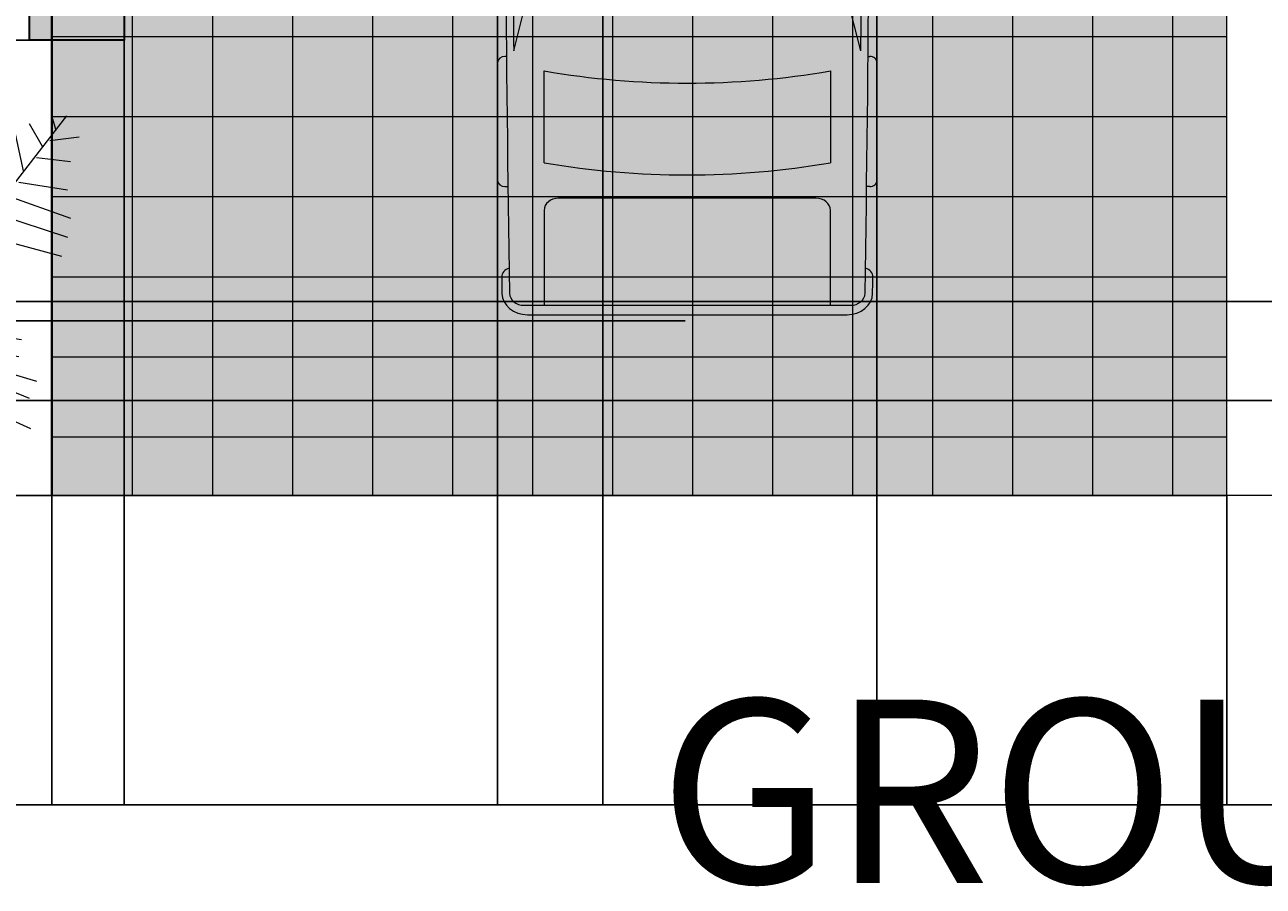
# Model space of a CAD drawing. Units: millimetres. Extents: x -229 to 16545, y -10488 to 4272.
# Tile 1 of 29: x 1930 to 5862, y -10488 to -7754. Entities that reach past the tile are written whole.
import ezdxf

# ---------------------------------------------------------------- set-up
doc = ezdxf.new("R2010")
doc.units = ezdxf.units.MM
for name, color, linetype, lineweight in [('A-ANNO-DIMS', 2, 'Continuous', 18), ('A-ANNO-TEXT', 7, 'Continuous', 25), ('A-COLS', 7, 'Continuous', 35), ('A-WALL', 7, 'Continuous', 35), ('C-PRKG-VEHI', 8, 'Continuous', 18), ('C-PRKG-VEHI-PATT', 252, 'Continuous', 13), ('L-PLNT-TREE', 80, 'Continuous', 18), ('L-PVMT', 7, 'Continuous', 18), ('L-PVMT-JNTS', 8, 'Continuous', 13)]:
    doc.layers.add(name, color=color, linetype=linetype, lineweight=lineweight)
doc.layers.add('L-PVMT-PATT', color=252, linetype='Continuous', lineweight=13, true_color=0x939598)
doc.styles.get("Standard").update_dxf_attribs({"font": 'arial.ttf'})
doc.dimstyles.get("Standard").update_dxf_attribs({"dimtxt": 0.18, "dimasz": 0.18, "dimexe": 0.18, "dimexo": 0.0625, "dimgap": 0.09, "dimtad": 0, "dimtih": 1, "dimtoh": 1, "dimdec": 4, "dimzin": 0, "dimdsep": 46, "dimtxsty": 'Standard', "dimcen": 0.09, "dimadec": 0, "dimazin": 0, "dimtfac": 1, "dimtdec": 4, "dimtofl": 0, "dimtmove": 0, "dimatfit": 3, "dimfxl": 1, "dimtolj": 1, "dimtzin": 0, "dimarcsym": 0})

# ---------------------------------------------------------------- blocks, each defined once
blk = doc.blocks.new('*U18')
for p, q in [((-10.18600000000015, 53.63999999999987), (-13.08399999999983, 55.96199999999976)), ((0, 0), (-10.5, 57)), ((-9.098999999999705, 51.7819999999997), (-6.563000000000101, 55.96199999999976)), ((-8.736999999999625, 47.13799999999969), (-17.06899999999996, 52.71100000000001)), ((-7.65000000000009, 43.42299999999977), (-2.577999999999974, 49.45999999999981)), ((-7.28800000000001, 39.70699999999965), (-21.77800000000025, 46.67299999999977)), ((-5.838999999999941, 35.99199999999973), (4.666999999999916, 48.06699999999977)), ((-5.114000000000032, 27.63199999999983), (10.46300000000019, 46.67299999999977)), ((-5.114000000000032, 28.09699999999975), (-24.67599999999993, 40.63599999999996)), ((-2.940999999999803, 16.48599999999987), (8.652000000000044, 37.84999999999991)), ((-3.665000000000418, 19.27299999999968), (-27.57400000000007, 35.52699999999982)), ((27, 9), (48, 36)), ((27.12699999999995, 9.05600000000004), (31.11200000000008, 35.99199999999973)), ((38.71900000000005, 34.13399999999979), (41.97899999999981, 28.56099999999992)), ((44.15300000000025, 36.45599999999991), (45.23900000000003, 32.74099999999999)), ((16.25900000000001, 5.804999999999836), (23.14199999999983, 31.34799999999973)), ((22.05499999999984, 7.197999999999865), (27.48900000000003, 32.27699999999982)), ((31.83600000000024, 30.88299999999981), (32.56100000000015, 16.48599999999987)), ((35.09600000000001, 32.74099999999999), (37.26999999999998, 22.52399999999989)), ((43.79100000000017, 29.95399999999995), (51.03600000000006, 30.88299999999981)), ((-48.58500000000003, 21.13099999999986), (-49.30899999999974, 29.02600000000007)), ((-43.51299999999992, 28.56099999999992), (-42.42699999999968, 15.55799999999976)), ((-35.54399999999987, 28.09699999999975), (-24.31399999999985, 3.946999999999661)), ((-31.5, 4.5), (-52.5, 25.5)), ((-38.44199999999955, 26.23899999999981), (-34.81899999999996, 7.662999999999783)), ((-14.5329999999999, 2.089999999999918), (-30.83399999999983, 25.30999999999995)), ((-1.128999999999905, 6.733999999999923), (9.014000000000124, 26.70399999999995)), ((3.942000000000007, 1.625), (11.1869999999999, 24.38099999999986)), ((10.10100000000011, 3.482999999999719), (17.70800000000008, 26.23899999999981)), ((40.52999999999975, 25.77499999999986), (48.86200000000008, 24.846)), ((-24.31399999999985, 23.91699999999969), (-2.940999999999803, 13.69999999999982)), ((-47.49800000000004, 19.73699999999962), (-55.83000000000038, 18.34399999999982)), ((36.18300000000045, 19.73699999999962), (48.13699999999972, 17.87999999999988)), ((33.28499999999986, 16.48599999999987), (48.86200000000008, 10.91299999999978)), ((-40.61500000000023, 13.69999999999982), (-55.10500000000002, 10.91299999999978)), ((-20.69099999999981, 13.69999999999982), (-1.128999999999905, 4.875999999999976)), ((29.66199999999981, 12.30699999999979), (48.13699999999972, 6.268999999999778)), ((-33.37000000000035, 6.268999999999778), (-52.20699999999988, 5.339999999999918)), ((0, 0), (27, 9)), ((24.22899999999982, 7.662999999999783), (46.6880000000001, 1.625)), ((-28.29899999999998, 3.482999999999719), (-47.86000000000012, -5.805000000000063)), ((0, 0), (-31.5, 4.5)), ((11.1869999999999, 3.482999999999719), (30.74900000000025, -5.805000000000063)), ((18.06999999999971, 5.804999999999836), (35.09600000000001, -3.483000000000174)), ((-21.41600000000017, 3.017999999999801), (-38.07899999999973, -8.128000000000384)), ((-15.98199999999951, 2.089999999999918), (-30.11000000000013, -9.521000000000186)), ((0, 0), (-22.5, -19.5)), ((-6.563000000000101, 1.161000000000058), (-21.41600000000017, -8.128000000000384)), ((0, 0), (18, -22.5)), ((6.478000000000065, 1.625), (26.03999999999996, -8.592000000000326)), ((2.493000000000392, -3.019000000000005), (-1.490999999999985, -20.20200000000023)), ((1.769000000000232, -2.555000000000063), (24.22899999999982, -9.521000000000186)), ((-6.563000000000101, -5.805000000000063), (-19.96699999999964, -9.985000000000127)), ((-4.751999999999952, -3.483000000000174), (-3.665000000000418, -14.62900000000013)), ((-9.460999999999785, -8.592000000000326), (-6.201000000000021, -23.4530000000002)), ((5.028999999999996, -6.270000000000209), (2.131000000000312, -25.77500000000009)), ((7.564999999999599, -9.056000000000267), (32.19800000000032, -14.62900000000013)), ((-13.44599999999991, -11.37800000000038), (-8.736999999999625, -32.74100000000021)), ((9.014000000000124, -11.37800000000038), (3.579999999999927, -35.99200000000019)), ((-17.43100000000004, -15.09400000000005), (-42.78899999999976, -18.80899999999997)), ((-15.2569999999996, -12.77200000000016), (-30.11000000000013, -12.77200000000016)), ((-17.06899999999996, -15.09400000000005), (-12.721, -40.17200000000025)), ((12.27399999999988, -15.09400000000005), (36.9069999999997, -18.80899999999997)), ((14.08499999999958, -16.95100000000025), (6.478000000000065, -40.17200000000025)), ((-22.5, -19.5), (-37.5, -45)), ((-20.69099999999981, -18.34500000000003), (-17.79300000000012, -44.35200000000032)), ((16.25900000000001, -19.73800000000028), (36.18300000000045, -22.98900000000003)), ((-24.31399999999985, -21.59600000000023), (-42.42699999999968, -22.06000000000017)), ((-25.03800000000001, -23.91800000000035), (-22.86500000000024, -45.28100000000017)), ((18.06999999999971, -22.52400000000012), (8.289000000000215, -45.74500000000012)), ((18, -22.5), (27, -52.5)), ((18.43300000000045, -22.52400000000012), (40.52999999999975, -29.02600000000007)), ((-26.8489999999997, -26.24000000000001), (-40.25300000000015, -25.77500000000009)), ((19.1569999999997, -25.31100000000015), (38.71900000000005, -33.20600000000013)), ((-28.29899999999998, -29.02600000000007), (-42.78899999999976, -31.34800000000018)), ((-29.02300000000014, -30.88400000000002), (-27.93600000000015, -43.88700000000016)), ((20.24400000000014, -30.4190000000001), (15.89699999999993, -44.81600000000026)), ((21.33100000000013, -32.74100000000021), (39.08100000000013, -40.63600000000019)), ((-30.83399999999983, -34.13499999999999), (-42.42699999999968, -35.52800000000025)), ((-32.64600000000019, -36.92100000000005), (-31.92099999999982, -44.35200000000032)), ((22.77999999999975, -37.85000000000014), (19.51900000000023, -48.53200000000015)), ((22.77999999999975, -38.31400000000008), (34.37199999999985, -44.81600000000026)), ((-34.45699999999988, -39.70800000000031), (-40.97800000000006, -42.49400000000014)), ((24.59100000000035, -43.42300000000022), (30.74900000000025, -47.60300000000029)), ((24.59100000000035, -45.74500000000012), (23.14199999999983, -50.85400000000004)), ((26.76400000000012, -49.92500000000018), (28.21300000000019, -50.85400000000004))]:
    blk.add_line(p, q)
blk = doc.blocks.new('*U20')
for p, q in [((46.55368679439944, 38.88847654282876), (22.35054758993934, 38.88847654282876)), ((136.6978032355602, 38.88847654282876), (160.90094244002, 38.88847654282867)), ((21.10406751471477, 37.40863046792069), (21.10406751471477, 36.83230215753705)), ((47.80016686962392, 37.39011648242055), (47.80016686962392, 37.40863046792069)), ((87.98532186932616, 31.87120872459877), (74.75900729854769, 35.92175679182955)), ((134.313356548143, 35.6043097713567), (119.2882629232503, 31.77757799177584)), ((135.4513231603356, 37.07354110333037), (135.4513231603356, 37.40863046792069)), ((162.1474225152445, 37.40863046792049), (162.1474225152445, 36.77402019194128)), ((186.4728846989705, -33.49860931502491), (186.4728846989718, 33.49860931502465)), ((70.0302824853563, 31.53613089391356), (86.40615155322342, 29.35124891408057)), ((188.3990091454065, -32.75868627757393), (188.3990091454077, 32.75868627757058)), ((138.4228833961707, 29.35124891408074), (157.2465674415997, 29.35124891408074)), ((186.4728846989718, 29.35124891408083), (167.0083537481071, 29.35124891408083)), ((164.515393597658, 26.39155676426461), (164.5153935976578, -26.39155676426503)), ((32.26591480791686, 11.62530558863241), (36.12873726252356, 17.16961494239206)), ((36.12873726252356, 17.16961494239206), (50.93891189819171, 17.16961494239206)), ((32.12291633764599, 9.505833383620029), (32.12291633764599, 11.15369945057711)), ((58.9167604809788, -10.77488335095668), (58.9167604809788, 10.77488335095617)), ((66.55009204259746, -10.5288681329018), (66.55009204259746, 10.52886813290129)), ((186.4728846989718, -10.5288681329018), (186.4728846989718, 10.52886813290129)), ((29.77279020470884, 9.505833383620029), (51.68362801571248, 9.505833383620029)), ((82.73706193978568, 8.496039918672748), (82.73706193978568, -8.49603991867258)), ((3.266462181856987, 6.128290093440767), (0.1022408397004821, 0.4060708604429806)), ((-4.43e-14, -2.558e-13), (51.68362801571248, -2.558e-13)), ((0.1022408397004821, -0.4060708604432933), (3.266462181856987, -6.128290093441194)), ((29.77279020470884, -9.50583338362054), (51.68362801571248, -9.50583338362054)), ((32.12291633764599, -9.50583338362054), (32.12291633764599, -11.15369945057762)), ((32.26591480791686, -11.62530558863292), (36.12873726252356, -17.16961494239257)), ((36.12873726252356, -17.16961494239257), (50.93891189819171, -17.16961494239257)), ((86.40615155322318, -29.35124891408145), (70.03028248535594, -31.53613089391442)), ((157.2465674415997, -29.35124891408117), (138.4228833961707, -29.35124891408126)), ((167.008353748107, -29.35124891408126), (186.4728846989707, -29.35124891408108)), ((87.98532186932607, -31.87120872459903), (74.7590072985476, -35.92175679182964)), ((134.3133565481428, -35.60430977135721), (119.2882629232503, -31.77757799177618)), ((21.10406751471477, -37.4086304679212), (21.10406751471477, -36.83230215753756)), ((47.80016686962392, -37.39011648242107), (47.80016686962392, -37.4086304679212)), ((135.4513231603355, -37.07354110333088), (135.4513231603355, -37.4086304679212)), ((162.1474225152445, -37.408630467921), (162.1474225152445, -36.77402019194179)), ((46.55368679439944, -38.88847654282927), (22.35054758993934, -38.88847654282927)), ((136.6978032355602, -38.88847654282927), (160.9009424400199, -38.88847654282918))]:
    blk.add_line(p, q)
for centre, major_axis, ratio, start_param, end_param in [((22.35054758993934, 37.40863046792072), (2.08e-14, -1.479846074908118), 0.842303869543976, 3.141592653589776, 4.712388980384677), ((46.55368679439944, 37.40863046792072), (2.2e-14, 1.479846074908118), 0.8423038695439758, -1.570796326794884, 1.73e-14), ((136.6978032355602, 37.40863046792072), (2.357e-13, -1.479846074908118), 0.842303869543976, 3.141592653589603, 4.712388980384554), ((160.90094244002, 37.40863046792052), (5.59e-14, 1.479846074908118), 0.842303869543976, -1.570796326794865, 4.44e-14), ((266.0300214172791, -27.52442688366631), (1.966072e-10, 313.3077612809058), 0.8423038695435284, 1.367075990158062, 1.391760499156098), ((41.19115208863305, -490.8631038926156), (1.294e-13, 528.2339998381949), 0.8423038695439741, 0.0028100083536837, 0.0755983031096952), ((64.48199294511879, -10555.61767587835), (1.907644e-10, 10593.02630634627), 0.842303869543847, -0.0133969486112073, 0.0027970409639888), ((64.4819929449925, -10555.61767590795), (1.9177683e-09, -10591.54646030096), 0.8423038695482963, 3.133765086725325, 3.140440689641252), ((180.6280394947615, 35.8381667808375), (7.4e-14, 2.219769112362114), 0.8423038695439693, -0.0130174256259048, 1.249894140392862), ((64.48199294754608, -10556.35759891604), (1.349839377e-06, 10595.3130398087), 0.8423038681351469, -0.0133969484821159, -0.0130174254969711), ((183.9799245485226, 33.49860931502124), (3e-16, -2.959692149816168), 0.8423038695439952, 1.570796326796048, 3.128195704978389), ((183.9799245485216, 32.75868627756583), (8.56e-14, -5.246425615115243), 0.8423038695439737, 1.570796326795794, 3.128195704978164), ((135.2911776514449, 5.387441675478555), (2.2715e-12, 81.77258453065997), 0.8423038695439563, 1.245306111696802, 1.507880129813836), ((95.78879860270445, -3666.353346297651), (1.949864e-10, -3698.236159209632), 0.8423038695446962, 3.134048706297306, 3.14409775411291), ((259.1750197310735, -27.52442688366614), (1.506617e-10, -305.3028914627677), 0.8423038695443789, 4.528606069860317, 4.561837674556238), ((37.47375371777758, -593.9621830607928), (6.21e-14, -623.32820996736), 0.8423038695439826, 3.09604606856106, 3.200911180495224), ((134.4003789125686, 5.387441675477674), (4.276e-13, -89.7774543484738), 0.84230386954398, 4.44948196380473, 4.652344057257214), ((149.595361812917, 2.799442537139299), (8.561e-13, -79.57966406425402), 0.842303869543983, 4.372215489277867, 4.640744122441986), ((17.08207736189386, -1.421e-13), (6.87e-14, 147.0179238898305), 0.8423038695439764, 4.511394369635731, 4.913383591133647), ((35.90576140732288, -1.421e-13), (6.87e-14, 147.0179238898305), 0.8423038695439764, 4.511394369635731, 4.913383591133647), ((167.0083537481071, 26.39155676426464), (1.394e-13, 2.959692149816236), 0.842303869543976, 5.55e-14, 1.57079632679492), ((-204.4946649195746, 52.39684969293512), (4.12053e-11, -250.9602162198571), 0.8423038695441164, 1.385369446298923, 1.434372047871027), ((13.03653510440275, 17.00972444508943), (1.2303e-12, 27.41599049210566), 0.8423038695439277, 4.435146050259648, 4.718221029521873), ((14.20086229321332, 17.00972444508943), (1.2303e-12, 27.41599049210566), 0.8423038695439277, 4.435146050259648, 4.718221029521873), ((50.7902773840875, 13.33772416300607), (6.340077547122382, -0.356608581037027), 0.6038335755719145, -1.39555193967809, 1.581314658479915), ((32.74615637525823, 11.15369945057713), (1.313e-13, 0.7399230374541176), 0.8423038695439091, 0.8797135699495516, 1.570796326795045), ((29.77279020470884, -46.66302566589627), (5.12e-14, 56.16885904951626), 0.842303869543976, 7e-16, 0.5903187773915901), ((0.6232400376122422, -1.421e-13), (1e-16, -0.7399230374541245), 0.842303869543842, 4.131459131953847, 5.293318828815531), ((29.77279020470884, 46.66302566589578), (4.004e-13, 56.16885904951626), 0.8423038695439734, 2.55127387619821, 3.141592653589801), ((-204.4946649195746, -52.39684969293552), (4.02945e-11, 250.9602162198562), 0.8423038695441192, -1.43437204787103, -1.385369446298926), ((13.03653510440275, -17.00972444508983), (1.2568e-12, -27.41599049210552), 0.8423038695439318, 1.564964277657711, 1.848039256919935), ((14.20086229321332, -17.00972444508983), (1.2568e-12, -27.41599049210552), 0.8423038695439318, 1.564964277657711, 1.848039256919935), ((149.5953618129329, -2.799442537137565), (4.0897e-12, -79.57966406427697), 0.8423038695439419, -1.499151468852248, -1.230622835688196), ((32.74615637525823, -11.1536994505777), (1.3e-13, -0.7399230374541176), 0.8423038695439093, 4.712388980384541, 5.403471737230034), ((134.4003789125684, -5.387441675478584), (4.2949e-12, -89.77745434847827), 0.8423038695439354, -1.510751403667474, -1.307889310215002), ((135.2911776514465, -5.387441675480715), (3.2038e-12, -81.77258453066244), 0.8423038695439492, -1.50788012981387, -1.245306111696839), ((259.1750197310694, 27.52442688365929), (1.08535e-11, 305.3028914629043), 0.8423038695439974, 1.721347632622872, 1.754579237318777), ((167.008353748107, -26.39155676426503), (1.02e-14, -2.959692149816192), 0.8423038695439885, 4.712388980384686, 6.283185307179581), ((266.0300214172791, 27.52442688366566), (8.75241e-11, 313.3077612806533), 0.8423038695441819, 1.749832154434603, 1.774516663432659), ((37.47375371777847, 593.9621830607904), (1.1693e-12, -623.3282099673584), 0.8423038695439528, -0.0593185269054384, 0.0455465850287298), ((95.78879860271888, 3666.35334629765), (1.637818e-10, -3698.236159209629), 0.8423038695447546, -0.0025051005232382, 0.007543947292366), ((183.9799245485177, -32.7586862775633), (2.428e-13, -5.246425615118353), 0.8423038695439808, 0.0133969486110846, 1.570796326792831), ((183.9799245485216, -33.4986093150211), (9.3e-15, 2.959692149816141), 0.8423038695439732, 3.154989602201626, 4.71238898038339), ((41.19115208863322, 490.8631038926152), (1.37757e-11, -528.2339998381949), 0.8423038695440652, -0.0755983031097181, -0.0028100083537155), ((22.35054758993934, -37.40863046792117), (2.2e-14, 1.479846074908118), 0.8423038695439758, 1.570796326794908, 3.14159265358981), ((64.48199294495228, 10555.61767590795), (6.117947e-10, 10593.02630637587), 0.8423038695458146, 3.138795612625926, 3.154989602201039), ((46.55368679439944, -37.40863046792117), (2.08e-14, -1.479846074908118), 0.842303869543976, -1.69e-14, 1.570796326794884), ((64.48199294503607, 10555.61767590793), (1.6049794e-09, -10591.54646030094), 0.8423038695397146, 0.0011519639481523, 0.0078275668641468), ((136.6978032355602, -37.40863046792109), (1.56e-14, -1.479846074908162), 0.8423038695440105, -1.570796326794875, -1.27e-14), ((160.9009424400199, -37.408630467921), (1.969e-13, 1.479846074908162), 0.8423038695440109, 3.141592653589951, 4.712388980384771), ((180.6280394947581, -35.83816678083949), (2.274e-13, -2.219769112363032), 0.8423038695439803, -1.249894138785958, 0.0130174256254374), ((64.48199294197605, 10556.3575989598), (9.365289701e-07, 10595.31303985772), 0.8423038705260315, 3.154610079306566, 3.154989602290631)]:
    blk.add_ellipse(centre, major_axis=major_axis, ratio=ratio, start_param=start_param, end_param=end_param)
at = {"extrusion": (0, 0, -1)}
blk.add_ellipse((50.7902773840875, -13.33772416300655), major_axis=(6.340077547122382, 0.3566085810370246), ratio=0.6038335755719145, start_param=-1.39555193967809, end_param=1.581314658479915, dxfattribs=at)
blk = doc.blocks.new('COL-300x450')
at = {"transparency": 33554615}
h = blk.add_hatch(color=256, dxfattribs=at)
h.dxf.hatch_style = 1
h.paths.add_polyline_path([(300, 450), (0, 450), (0, 0), (300, 0)])
at = {"transparency": 33554687}
blk.add_lwpolyline([(0, 450), (300, 450), (300, 0), (0, 0)], close=True, dxfattribs=at)
blk = doc.blocks.new('*D47')
at = {"layer": 'A-ANNO-DIMS', "color": 0, "lineweight": -2, "transparency": 16777216}
for p, q in [((912.052246, -9248.334552), (912.0522459999999, -10230.221103)), ((15679.60703, -9248.334552), (15679.60703, -10230.221103)), ((912.2322459999997, -10230.041103), (8295.409228723058, -10230.041103)), ((15679.42703, -10230.041103), (8296.250047276942, -10230.041103))]:
    blk.add_line(p, q, dxfattribs=at)
at = {"layer": 'A-ANNO-DIMS', "color": 0, "transparency": 16777216}
for points in [[(912.2322459999997, -10230.011103), (912.2322459999997, -10230.071103), (912.0522459999999, -10230.041103)], [(15679.42703, -10230.011103), (15679.42703, -10230.071103), (15679.60703, -10230.041103)]]:
    blk.add_solid(points, dxfattribs=at)
at = {"layer": 'Defpoints', "color": 0, "transparency": 16777216}
for p in [(912.052246, -9248.272052), (15679.60703, -9248.272052), (15679.60703, -10230.041103)]:
    blk.add_point(p, dxfattribs=at)
at = {"layer": 'A-ANNO-DIMS', "color": 0, "transparency": 16777216, "insert": (8295.829637999997, -10230.041103), "char_height": 0.18, "attachment_point": 5}
blk.add_mtext('\\A1;14768', dxfattribs=at)
blk = doc.blocks.new('*D58')
at = {"layer": 'A-ANNO-DIMS', "color": 0, "lineweight": -2, "transparency": 16777216}
for p, q in [((2015.933029, -9248.334552), (2015.933029, -10230.221103)), ((5745.933028999999, -9248.334552), (5745.933028999999, -10230.221103)), ((2016.113029, -10230.041103), (3880.574625180082, -10230.041103)), ((5745.753028999999, -10230.041103), (3881.291432819919, -10230.041103))]:
    blk.add_line(p, q, dxfattribs=at)
at = {"layer": 'A-ANNO-DIMS', "color": 0, "transparency": 16777216}
for points in [[(2016.113029, -10230.011103), (2016.113029, -10230.071103), (2015.933029, -10230.041103)], [(5745.753028999999, -10230.011103), (5745.753028999999, -10230.071103), (5745.933028999999, -10230.041103)]]:
    blk.add_solid(points, dxfattribs=at)
at = {"layer": 'Defpoints', "color": 0, "transparency": 16777216}
for p in [(2015.933029, -9248.272052), (5745.933028999999, -9248.272052), (5745.933028999999, -10230.041103)]:
    blk.add_point(p, dxfattribs=at)
at = {"layer": 'A-ANNO-DIMS', "color": 0, "transparency": 16777216, "insert": (3880.933029, -10230.041103), "char_height": 0.18, "attachment_point": 5}
blk.add_mtext('\\A1;3730', dxfattribs=at)
blk = doc.blocks.new('*D62')
at = {"layer": 'A-ANNO-DIMS', "color": 0, "lineweight": -2, "transparency": 16777216}
for p, q in [((5745.870529000002, -4748.272052000002), (-228.8374730000013, -4748.272052000003)), ((-228.6574730000007, -4748.452052000003), (-228.6574730000002, -6998.090148862215)), ((-228.6574729999998, -9248.092052000005), (-228.6574730000002, -6998.453955137795)), ((5745.870529000002, -9248.272052000004), (-228.8374730000003, -9248.272052000006))]:
    blk.add_line(p, q, dxfattribs=at)
at = {"layer": 'A-ANNO-DIMS', "color": 0, "transparency": 16777216}
for points in [[(-228.6874730000008, -4748.452052000003), (-228.6274730000008, -4748.452052000003), (-228.6574730000007, -4748.272052000003)], [(-228.6874729999997, -9248.092052000005), (-228.6274729999997, -9248.092052000005), (-228.6574729999998, -9248.272052000006)]]:
    blk.add_solid(points, dxfattribs=at)
at = {"layer": 'Defpoints', "color": 0, "transparency": 16777216}
for p in [(5745.933029000002, -4748.272052000002), (-228.6574729999998, -9248.272052000006), (5745.933029000002, -9248.272052000004)]:
    blk.add_point(p, dxfattribs=at)
at = {"layer": 'A-ANNO-DIMS', "color": 0, "transparency": 16777216, "insert": (-228.6574730000022, -6998.272052000003), "char_height": 0.18, "attachment_point": 5}
blk.add_mtext('\\A1;4500', dxfattribs=at)
blk = doc.blocks.new('*D91')
at = {"layer": 'A-ANNO-DIMS', "color": 0, "lineweight": -2, "transparency": 16777216}
for p, q in [((2245.933029, -4748.334552), (2245.933028999999, -10230.221103)), ((3765.491243, -4748.334552), (3765.491243, -10230.221103)), ((2246.113028999999, -10230.041103), (3005.257040502046, -10230.041103)), ((3765.311243, -10230.041103), (3006.167231497953, -10230.041103))]:
    blk.add_line(p, q, dxfattribs=at)
at = {"layer": 'A-ANNO-DIMS', "color": 0, "transparency": 16777216}
for points in [[(2246.113028999999, -10230.011103), (2246.113028999999, -10230.071103), (2245.933028999999, -10230.041103)], [(3765.311243, -10230.011103), (3765.311243, -10230.071103), (3765.491243, -10230.041103)]]:
    blk.add_solid(points, dxfattribs=at)
at = {"layer": 'Defpoints', "color": 0, "transparency": 16777216}
for p in [(2245.933029, -4748.272051999999), (3765.491243, -4748.272051999999), (3765.491243, -10230.041103)]:
    blk.add_point(p, dxfattribs=at)
at = {"layer": 'A-ANNO-DIMS', "color": 0, "transparency": 16777216, "insert": (3005.712136, -10230.041103), "char_height": 0.18, "attachment_point": 5}
blk.add_mtext('\\A1;1519.6', dxfattribs=at)
blk = doc.blocks.new('*D92')
at = {"layer": 'A-ANNO-DIMS', "color": 0, "lineweight": -2, "transparency": 16777216}
for p, q in [((1945.870529000001, -7803.015189000004), (-228.8374730000004, -7803.015189000004)), ((-228.6574730000004, -7803.195189000004), (-228.6574730000002, -8525.461655970674)), ((-228.6574730000001, -9248.092052000004), (-228.6574730000002, -8525.825585029335)), ((2015.870529000001, -9248.272052000004), (-228.8374729999999, -9248.272052000004))]:
    blk.add_line(p, q, dxfattribs=at)
at = {"layer": 'A-ANNO-DIMS', "color": 0, "transparency": 16777216}
for points in [[(-228.6874730000004, -7803.195189000004), (-228.6274730000004, -7803.195189000004), (-228.6574730000004, -7803.015189000004)], [(-228.6874730000001, -9248.092052000004), (-228.6274730000001, -9248.092052000004), (-228.6574730000001, -9248.272052000004)]]:
    blk.add_solid(points, dxfattribs=at)
at = {"layer": 'Defpoints', "color": 0, "transparency": 16777216}
for p in [(1945.933029000001, -7803.015189000004), (-228.6574730000001, -9248.272052000004), (2015.933029000001, -9248.272052000004)]:
    blk.add_point(p, dxfattribs=at)
at = {"layer": 'A-ANNO-DIMS', "color": 0, "transparency": 16777216, "insert": (-228.6574730000026, -8525.643620500003), "char_height": 0.18, "attachment_point": 5}
blk.add_mtext('\\A1;1445.3', dxfattribs=at)
blk = doc.blocks.new('*D95')
at = {"layer": 'A-ANNO-DIMS', "color": 0, "lineweight": -2, "transparency": 16777216}
for p, q in [((3431.620292, -6103.680351), (3431.620292, -10230.221103)), ((4635.562560999999, -6103.680351), (4635.562560999999, -10230.221103)), ((3431.800292, -10230.041103), (4033.241494712823, -10230.041103)), ((4635.382560999999, -10230.041103), (4033.941358287175, -10230.041103))]:
    blk.add_line(p, q, dxfattribs=at)
at = {"layer": 'A-ANNO-DIMS', "color": 0, "transparency": 16777216}
for points in [[(3431.800292, -10230.011103), (3431.800292, -10230.071103), (3431.620292, -10230.041103)], [(4635.382560999999, -10230.011103), (4635.382560999999, -10230.071103), (4635.562560999999, -10230.041103)]]:
    blk.add_solid(points, dxfattribs=at)
at = {"layer": 'Defpoints', "color": 0, "transparency": 16777216}
for p in [(3431.620292, -6103.617851), (4635.562560999999, -6103.617851), (4635.562560999999, -10230.041103)]:
    blk.add_point(p, dxfattribs=at)
at = {"layer": 'A-ANNO-DIMS', "color": 0, "transparency": 16777216, "insert": (4033.591426499999, -10230.041103), "char_height": 0.18, "attachment_point": 5}
blk.add_mtext('\\A1;1204', dxfattribs=at)
blk = doc.blocks.new('*D96')
at = {"layer": 'A-ANNO-DIMS', "color": 0, "lineweight": -2, "transparency": 16777216}
for p, q in [((4033.528927000001, -5757.644295000002), (-228.8374730000011, -5757.644295000003)), ((-228.6574730000006, -5757.824295000003), (-228.6574730000002, -7225.597539470673)), ((-228.6574729999999, -8693.734713000003), (-228.6574730000002, -7225.961468529336)), ((4027.243185000002, -8693.914713000004), (-228.837473, -8693.914713000004))]:
    blk.add_line(p, q, dxfattribs=at)
at = {"layer": 'A-ANNO-DIMS', "color": 0, "transparency": 16777216}
for points in [[(-228.6874730000005, -5757.824295000003), (-228.6274730000005, -5757.824295000003), (-228.6574730000006, -5757.644295000003)], [(-228.6874729999999, -8693.734713000003), (-228.6274729999999, -8693.734713000003), (-228.6574729999999, -8693.914713000004)]]:
    blk.add_solid(points, dxfattribs=at)
at = {"layer": 'Defpoints', "color": 0, "transparency": 16777216}
for p in [(4033.591427000001, -5757.644295000002), (-228.6574729999999, -8693.914713000004), (4027.305685000001, -8693.914713000004)]:
    blk.add_point(p, dxfattribs=at)
at = {"layer": 'A-ANNO-DIMS', "color": 0, "transparency": 16777216, "insert": (-228.6574730000022, -7225.779504000001), "char_height": 0.18, "attachment_point": 5}
blk.add_mtext('\\A1;2936', dxfattribs=at)
blk = doc.blocks.new('*D98')
at = {"layer": 'A-ANNO-DIMS', "color": 0, "lineweight": -2, "transparency": 16777216}
for p, q in [((5975.870529000001, -8632.301380000004), (-228.8374730000005, -8632.301380000006)), ((-228.6574730000003, -8632.481380000007), (-228.6574730000002, -8789.345922470675)), ((-228.6574730000002, -8946.574394000005), (-228.6574730000002, -8789.709851529336)), ((5975.870529000001, -8946.754394000001), (-228.8374730000004, -8946.754394000007))]:
    blk.add_line(p, q, dxfattribs=at)
at = {"layer": 'A-ANNO-DIMS', "color": 0, "transparency": 16777216}
for points in [[(-228.6874730000003, -8632.481380000007), (-228.6274730000003, -8632.481380000007), (-228.6574730000003, -8632.301380000006)], [(-228.6874730000002, -8946.574394000005), (-228.6274730000002, -8946.574394000005), (-228.6574730000002, -8946.754394000007)]]:
    blk.add_solid(points, dxfattribs=at)
at = {"layer": 'Defpoints', "color": 0, "transparency": 16777216}
for p in [(-228.6574730000003, -8632.301380000006), (5975.933029000001, -8632.301380000004), (5975.933029000001, -8946.754394000001)]:
    blk.add_point(p, dxfattribs=at)
at = {"layer": 'A-ANNO-DIMS', "color": 0, "transparency": 16777216, "insert": (-228.6574730000027, -8789.527887000004), "char_height": 0.18, "attachment_point": 5}
blk.add_mtext('\\A1;314.45', dxfattribs=at)

msp = doc.modelspace()

# ---------------------------------------------------------------- hatches: boundary and pattern name
at = {"layer": 'C-PRKG-VEHI-PATT'}
h = msp.add_hatch(color=256, dxfattribs=at)
h.dxf.hatch_style = 1
edge = h.paths.add_edge_path()
edge.add_ellipse((3607.529211185457, -9769.523765348671), major_axis=(4725.912256580008, 3.0749239e-09), ratio=0.8423038695445281, start_angle=77.5553727065174, end_angle=79.7904610028182)
edge.add_ellipse((4844.664368095724, -2592.185106036592), major_axis=(3884.719060684347, 1.125906e-09), ratio=0.8423038695442183, start_angle=257.4450673558462, end_angle=260.74343399278183, ccw=False)
edge.add_line((4128.453814510914, -5808.20724164565), (4039.87716894264, -5759.226924584826))
edge.add_ellipse((4033.591426782733, -5767.29169096579), major_axis=(11.45358085171419, 4.4945e-12), ratio=0.8423038695438549, start_angle=52.06686954012766, end_angle=89.99999999999291)
edge.add_line((4033.59142678273, -5757.644295494259), (4033.59142678273, -5810.864491195777))
edge.add_ellipse((3311.274766540754, -6218.509875466019), major_axis=(-869.4614654596021, 1.80077e-11), ratio=0.8423038695439853, start_angle=180.0000000000011, end_angle=209.4385695979805, ccw=False)
edge.add_line((4180.736232000355, -6218.50987546602), (4180.736232000355, -6254.888469336996))
edge.add_line((4180.736232000355, -6254.888469336996), (4208.936604088284, -6254.888469336996))
edge.add_ellipse((4206.244246044127, -6264.535864808529), major_axis=(-11.45358085171833, 5.0922e-12), ratio=0.8423038695436069, start_angle=225.5197891174528, end_angle=270.00000000002547, ccw=False)
edge.add_line((4213.544436413884, -6257.102002985786), (4299.367139905714, -6316.896261388502))
edge.add_line((4299.367139905714, -6316.896261388502), (4299.367139905714, -6546.149202615045))
edge.add_ellipse((4240.051685953036, -6543.848426266054), major_axis=(5.520094670108304, 98.1407350715287), ratio=0.6038335755718915, start_angle=106.3425919543132, end_angle=270.99798572498946, ccw=False)
edge.add_line((4180.736232000355, -6557.67697757519), (4180.736232000355, -6218.50987546602))
edge.add_ellipse((3311.274766540754, -6218.509875466019), major_axis=(-869.4614654596021, 1.80077e-11), ratio=0.8423038695439853, start_angle=180.0000000000011, end_angle=209.4385695979805)
edge.add_ellipse((4755.908087024709, -6218.50987546602), major_axis=(869.4614654596019, 1.2409e-11), ratio=0.842303869543984, start_angle=150.5614304020198, end_angle=179.9999999999992)
edge.add_line((3886.446621565107, -6218.509875466021), (3886.446621565105, -6557.676977575214))
edge.add_ellipse((3827.131167612427, -6543.848426266054), major_axis=(-5.520094670108304, 98.1407350715287), ratio=0.6038335755718915, start_angle=89.0020142750106, end_angle=253.6574080456868, ccw=False)
edge.add_line((3767.815713659748, -6546.149202615045), (3767.815713659748, -6316.896261388502))
edge.add_line((3767.815713659748, -6316.896261388502), (3855.713030733728, -6255.656581488097))
edge.add_ellipse((3860.938607521334, -6264.535864808529), major_axis=(-11.45358085171114, 2.4167e-12), ratio=0.842303869544136, start_angle=-89.99999999998789, end_angle=-45.51978911742532, ccw=False)
edge.add_line((3860.938607521328, -6254.888469336996), (3886.446621565107, -6254.888469336996))
edge.add_line((3886.446621565107, -6254.888469336996), (3886.446621565107, -6218.509875466018))
edge.add_ellipse((4755.908087024709, -6218.50987546602), major_axis=(869.4614654596019, 1.2409e-11), ratio=0.842303869543984, start_angle=150.5614304020199, end_angle=179.9999999999992, ccw=False)
edge.add_line((4033.59142678273, -5810.86449119578), (4033.59142678273, -5757.644295494258))
edge.add_ellipse((4033.591426782733, -5767.29169096579), major_axis=(11.45358085171419, 4.4945e-12), ratio=0.8423038695438549, start_angle=89.99999999999291, end_angle=127.9331304598159)
edge.add_line((4027.305684622828, -5759.226924584826), (3938.729039054555, -5808.207241645646))
edge.add_ellipse((3222.518485469741, -2592.185106036592), major_axis=(3884.719060685492, 7.18321e-11), ratio=0.8423038695439776, start_angle=-80.74343399279951, end_angle=-77.44506735586378, ccw=False)
edge.add_ellipse((4459.653642379904, -9769.523765348607), major_axis=(4725.912256583255, 9.99789e-11), ratio=0.8423038695439494, start_angle=100.2095389971419, end_angle=102.4446272934428)
edge.add_ellipse((13227.78263612094, -6337.716338528086), major_axis=(9648.760328614822, 3.05852e-11), ratio=0.8423038695439373, start_angle=177.1362853921621, end_angle=182.1985405659548)
edge.add_ellipse((3950.196944261551, -7838.084460829144), major_axis=(1389.703090715241, 7.69205e-11), ratio=0.842303869543924, start_angle=94.082410691147, end_angle=107.71995322274691, ccw=False)
edge.add_line((3866.802461740376, -6669.641686482127), (4200.380391825095, -6669.641686482127))
edge.add_ellipse((4116.985909303905, -7838.084460829148), major_axis=(1389.703090715146, 5.3309e-12), ratio=0.8423038695439844, start_angle=72.28004677724942, end_angle=85.91758930884919, ccw=False)
edge.add_ellipse((-5160.599782555511, -6337.716338528068), major_axis=(9648.76032861485, 3.05852e-11), ratio=0.8423038695439409, start_angle=-2.198540565955437, end_angle=2.863714607837381)
edge = h.paths.add_edge_path()
edge.add_ellipse((-159361.2677283546, -6755.788267626439), major_axis=(-163973.9231279127, 1.03867551e-08), ratio=0.8423038695433289, start_angle=179.6161332212111, end_angle=180.0902290885979)
edge.add_ellipse((-159361.2677283546, -6755.788267626439), major_axis=(-163973.9231279127, 1.03867551e-08), ratio=0.8423038695433289, start_angle=180.0902290885979, end_angle=180.1349865768619)
edge.add_ellipse((-3564.68564119695, -6395.259516187628), major_axis=(-8176.756932164527, 2.256357e-10), ratio=0.8423038695440322, start_angle=180.1356123904399, end_angle=182.1799503136467)
edge.add_ellipse((-3564.68564119695, -6395.259516187628), major_axis=(-8176.756932164527, 2.256357e-10), ratio=0.8423038695440322, start_angle=182.1799503136467, end_angle=183.6504275857005)
edge.add_ellipse((3607.529211185454, -9875.635228402642), major_axis=(4849.823013544719, 2.3877334e-09), ratio=0.8423038695443318, start_angle=76.21947101047385, end_angle=77.87403444768762)
edge.add_ellipse((-5160.599782555511, -6337.716338528068), major_axis=(9648.76032861485, 3.05852e-11), ratio=0.8423038695439409, start_angle=-2.1985405659553976, end_angle=2.8637146078373803, ccw=False)
edge.add_ellipse((4116.985909303905, -7838.084460829148), major_axis=(1389.703090715146, 5.3309e-12), ratio=0.8423038695439844, start_angle=72.28004677724944, end_angle=85.91758930884916)
edge.add_line((4200.380391825095, -6669.641686482127), (3866.802461740375, -6669.641686482127))
edge.add_ellipse((3950.196944261551, -7838.084460829144), major_axis=(1389.703090715241, 7.69205e-11), ratio=0.842303869543924, start_angle=94.08241069114707, end_angle=107.7199532227469)
edge.add_ellipse((13227.78263612094, -6337.716338528086), major_axis=(9648.760328614822, 3.05852e-11), ratio=0.8423038695439373, start_angle=177.1362853921622, end_angle=182.1985405659549, ccw=False)
edge.add_ellipse((4459.653642380003, -9875.635228402642), major_axis=(4849.823013547592, 8.133391e-10), ratio=0.8423038695438513, start_angle=102.1259655522744, end_angle=103.7805289894881)
edge.add_ellipse((11631.86849476242, -6395.259516187635), major_axis=(8176.756932164531, 1.784299e-10), ratio=0.8423038695440094, start_angle=176.3495724142996, end_angle=177.8200496863535)
edge.add_ellipse((11631.86849476242, -6395.259516187635), major_axis=(8176.756932164531, 1.784299e-10), ratio=0.8423038695440094, start_angle=177.8200496863535, end_angle=179.8643876095602)
edge.add_ellipse((167428.4505823782, -6755.788267623933), major_axis=(-163973.9231283709, 3.9422692e-09), ratio=0.8423038695444919, start_angle=-0.1349865768556417, end_angle=-0.0902290885918171)
edge.add_ellipse((167428.4505823782, -6755.788267623933), major_axis=(-163973.9231283709, 3.9422692e-09), ratio=0.8423038695444919, start_angle=-0.0902290885918171, end_angle=0.3838667787936917)
edge.add_ellipse((167428.4505823782, -6755.788267623933), major_axis=(-163973.9231283709, 3.9422692e-09), ratio=0.8423038695444919, start_angle=0.3838667787936917, end_angle=0.5282714718187317)
edge.add_ellipse((167428.4505823782, -6755.788267623933), major_axis=(-163973.9231283709, 3.9422692e-09), ratio=0.8423038695444919, start_angle=0.5282714718187317, end_angle=0.6465540970623085)
edge.add_ellipse((3515.052320972862, -8605.547164094223), major_axis=(45.81432340685111, 4.6009e-12), ratio=0.8423038695439874, start_angle=180.6465540970845, end_angle=269.9999999999056)
edge.add_line((3515.052320972781, -8644.136745980357), (3579.251062286293, -8644.136745980357))
edge.add_line((3579.251062286293, -8644.136745980357), (3579.25106228629, -8338.779260567762))
edge.add_ellipse((3625.065385693143, -8342.837059794769), major_axis=(-45.81432340685263, 1.5796e-12), ratio=0.8423038695439878, start_angle=-89.9999999999979, end_angle=1.9895196601282805e-12, ccw=False)
edge.add_line((3625.065385693143, -8304.247477908637), (4446.934968270596, -8304.247477908639))
edge.add_ellipse((4442.11746787232, -8342.837059794772), major_axis=(-45.81432340685263, 2.8e-15), ratio=0.842303869543988, start_angle=180, end_angle=270, ccw=False)
edge.add_line((4487.931791279172, -8342.837059794772), (4487.931791279172, -8644.136745980375))
edge.add_line((4487.931791279172, -8644.136745980373), (4552.130532592662, -8644.136745980375))
edge.add_ellipse((4552.130532592609, -8605.547164094241), major_axis=(-45.81432340685346, 1.7729e-12), ratio=0.8423038695439725, start_angle=90.000000000083, end_angle=179.3534459029321)
edge.add_ellipse((-159361.2677283546, -6755.788267626439), major_axis=(-163973.9231279127, 1.03867551e-08), ratio=0.8423038695433289, start_angle=179.3534459029417, end_angle=179.3813568036844)
edge.add_ellipse((-159361.2677283546, -6755.788267626439), major_axis=(-163973.9231279127, 1.03867551e-08), ratio=0.8423038695433289, start_angle=179.3813568036844, end_angle=179.4717285281857)
edge.add_ellipse((-159361.2677283546, -6755.788267626439), major_axis=(-163973.9231279127, 1.03867551e-08), ratio=0.8423038695433289, start_angle=179.4717285281857, end_angle=179.6161332212111)
edge = h.paths.add_edge_path(flags=16)
edge.add_ellipse((-52719.43876303247, -7240.399519955929), major_axis=(57246.55770143846, 8.170279e-10), ratio=0.842303869544162, start_angle=-0.3640763488911554, end_angle=0.1208973690318383)
edge.add_line((4526.939312293975, -7119.606211509014), (4589.639454651214, -6914.870508417749))
edge.add_ellipse((-159361.2677288128, -6755.788267624483), major_axis=(163951.0159666675, 3.23007761e-08), ratio=0.842303869549042, start_angle=-0.37776419392122307, end_angle=-0.055594313510596294, ccw=False)
edge.add_line((4584.725558298378, -7836.737404937529), (4525.48996268015, -7604.157642007916))
edge = h.paths.add_edge_path(flags=16)
edge.add_line((4165.105212949923, -7038.366181950441), (3902.077640615548, -7038.366181950441))
edge.add_ellipse((3990.257674735825, -8073.294011525872), major_axis=(1231.84719271423, 3.9463e-11), ratio=0.8423038695439561, start_angle=94.87006959713399, end_angle=112.7919148775847)
edge.add_line((3579.251062286288, -7095.161567973676), (3545.430352373573, -6841.672582103935))
edge.add_ellipse((3950.196944261518, -7851.873510313874), major_axis=(1265.792333751566, 7.14673e-11), ratio=0.8423038695439378, start_angle=94.2774209630507, end_angle=111.8349537967049, ccw=False)
edge.add_line((3870.610635088292, -6787.801246035458), (4196.572218477172, -6787.801246035458))
edge.add_ellipse((4116.985909303919, -7851.87351031385), major_axis=(1265.792333751468, 7.9473e-12), ratio=0.8423038695439835, start_angle=68.16504620328988, end_angle=85.72257903694413, ccw=False)
edge.add_line((4521.752501191884, -6841.672582103939), (4487.931791279168, -7095.16156797368))
edge.add_ellipse((4076.925178829671, -8073.294011525625), major_axis=(1231.847192713881, 3.61807e-11), ratio=0.8423038695439931, start_angle=67.20808512240832, end_angle=85.12993040286263)
edge = h.paths.add_edge_path(flags=16)
edge.add_ellipse((4033.591426782733, -6022.064977478797), major_axis=(-2275.752467063544, 5.6979e-12), ratio=0.8423038695439709, start_angle=76.4018653097695, end_angle=103.5981346902307)
edge.add_line((4487.931791279172, -7900.350504724528), (4487.931791279172, -8191.730251303665))
edge.add_ellipse((4033.591426782733, -6313.444724057934), major_axis=(2275.752467063524, 1.15e-12), ratio=0.8423038695439785, start_angle=256.4018653097693, end_angle=283.5981346902305, ccw=False)
edge.add_line((3579.25106228629, -8191.730251303662), (3579.25106228629, -7900.350504724527))
edge = h.paths.add_edge_path(flags=16)
edge.add_line((3541.69289088531, -7604.157642007925), (3482.457295267053, -7836.737404937647))
edge.add_ellipse((167428.450582378, -6755.788267625229), major_axis=(163951.0159666672, 1.7265743e-08), ratio=0.842303869542198, start_angle=180.055594313493, end_angle=180.3777641939035, ccw=False)
edge.add_line((3477.543398914246, -6914.870508417725), (3540.243541271509, -7119.606211509064))
edge.add_ellipse((60786.62161659793, -7240.399519956177), major_axis=(-57246.55770143843, 1.560408e-10), ratio=0.8423038695499789, start_angle=-0.1208973690328125, end_angle=0.364076348890219)
h = msp.add_hatch(color=256, dxfattribs=at)
h.dxf.hatch_style = 1
edge = h.paths.add_edge_path()
edge.add_ellipse((4116.985909303919, -7851.87351031385), major_axis=(1265.792333751468, 7.9473e-12), ratio=0.8423038695439835, start_angle=68.1650462032899, end_angle=85.72257903694413)
edge.add_line((4196.572218477172, -6787.801246035458), (3870.610635088292, -6787.801246035458))
edge.add_ellipse((3950.196944261518, -7851.873510313874), major_axis=(1265.792333751566, 7.14673e-11), ratio=0.8423038695439378, start_angle=94.27742096305064, end_angle=111.8349537967049)
edge.add_line((3545.430352373573, -6841.672582103933), (3579.251062286288, -7095.161567973675))
edge.add_ellipse((3990.257674735825, -8073.294011525872), major_axis=(1231.84719271423, 3.9463e-11), ratio=0.8423038695439561, start_angle=94.87006959713398, end_angle=112.79191487758479, ccw=False)
edge.add_line((3902.077640615549, -7038.366181950441), (4165.105212949924, -7038.366181950441))
edge.add_ellipse((4076.925178829671, -8073.294011525625), major_axis=(1231.847192713881, 3.61807e-11), ratio=0.8423038695439931, start_angle=67.2080851224083, end_angle=85.12993040286261, ccw=False)
edge.add_line((4487.931791279168, -7095.16156797368), (4521.752501191884, -6841.672582103939))
edge = h.paths.add_edge_path()
edge.add_ellipse((4033.591426782733, -6022.064977478797), major_axis=(-2275.752467063544, 5.6979e-12), ratio=0.8423038695439709, start_angle=76.4018653097695, end_angle=103.59813469023078, ccw=False)
edge.add_line((3579.25106228629, -7900.350504724527), (3579.25106228629, -8191.730251303662))
edge.add_ellipse((4033.591426782733, -6313.444724057934), major_axis=(2275.752467063524, 1.15e-12), ratio=0.8423038695439785, start_angle=256.4018653097692, end_angle=283.5981346902305)
edge.add_line((4487.931791279172, -8191.730251303665), (4487.931791279172, -7900.35050472453))
edge = h.paths.add_edge_path()
edge.add_ellipse((4442.11746787232, -8342.837059794772), major_axis=(-45.81432340685263, 2.8e-15), ratio=0.842303869543988, start_angle=180, end_angle=270)
edge.add_line((4442.117467872324, -8304.24747790864), (3625.065385693137, -8304.247477908639))
edge.add_ellipse((3625.065385693143, -8342.837059794769), major_axis=(-45.81432340685263, 1.5796e-12), ratio=0.8423038695439878, start_angle=-89.99999999999801, end_angle=1.9717e-12)
edge.add_line((3579.25106228629, -8342.837059794769), (3579.251062286293, -8644.136745980357))
edge.add_line((3579.251062286293, -8644.136745980357), (4487.931791279172, -8644.136745980371))
edge.add_line((4487.931791279172, -8644.136745980373), (4487.931791279172, -8342.837059794772))
at = {"layer": 'L-PVMT-JNTS', "transparency": 33554523}
h = msp.add_hatch(dxfattribs=at)
h.set_pattern_fill('NET', color=256, scale=80)
h.set_pattern_definition([(0, (-8141.222001159148, -13125.50409224634), (0, 254), []), (90, (-8141.222001159148, -13125.50409224634), (-254, 1.56e-14), [])])
h.paths.add_polyline_path([(5745.933029018122, -5438.272051523089), (5745.933029018122, -4748.272051523088), (2245.933029018121, -4748.272051523088), (2245.933029018121, -5217.29063777321), (2015.933029018121, -5217.29063777321), (2015.93302901812, -9248.272051523089), (5745.933029018122, -9248.272051523089)])
at = {"layer": 'L-PVMT-PATT', "transparency": 33554493}
h = msp.add_hatch(color=256, dxfattribs=at)
h.dxf.hatch_style = 1
h.paths.add_polyline_path([(5745.933029018122, -5438.272051523089), (5745.933029018122, -4748.272051523088), (2245.933029018121, -4748.272051523088), (2245.933029018121, -5217.29063777321), (2015.933029018121, -5217.29063777321), (2015.93302901812, -9248.272051523089), (5745.933029018122, -9248.272051523089)])

# ---------------------------------------------------------------- linework, layer by layer
at = {"layer": 'A-WALL'}
msp.add_line((2015.933029018121, -9248.272051523089), (2015.933029018121, 2251.727948476911), dxfattribs=at)
at = {"layer": 'L-PVMT'}
for p, q in [((5745.933029018122, -9248.272051523089), (5745.933029018122, -5438.272051523089)), ((2015.933029018121, -9248.272051523087), (2015.933029018121, -7805.231013702166)), ((2245.933029018121, -9248.272051523089), (2245.933029018121, -7803.015189216734)), ((14015.93302901812, -9248.272051523089), (2015.933029018121, -9248.272051523089))]:
    msp.add_line(p, q, dxfattribs=at)

# ---------------------------------------------------------------- block references
at = {"layer": 'A-COLS'}
msp.add_blockref('COL-300x450', (1945.93302901812, -7803.015189216731), dxfattribs=at)
at = {"layer": 'C-PRKG-VEHI', "xscale": 15.47942187490615, "yscale": 15.47942187490615, "zscale": 15.47942187490615, "rotation": 270}
msp.add_blockref('*U20', (4033.591426782735, -5757.644295494259), dxfattribs=at)
at = {"layer": 'L-PLNT-TREE', "xscale": 12.94000768461256, "yscale": 12.94000768461256, "zscale": 12.94000768461256}
msp.add_blockref('*U18', (1442.982306165615, -8509.019337727086), dxfattribs=at)

# ---------------------------------------------------------------- texts
at = {"layer": 'A-ANNO-TEXT'}
msp.add_text('GROUNDFLOOR PLAN', height=582.3251988104383, dxfattribs=at).set_placement((3943.488631400338, -10477.8144340376))

# ---------------------------------------------------------------- dimensions: what is measured, and where the dimension line sits
at = {"layer": 'A-ANNO-DIMS'}
for base, p1, p2, override, picture, middle in [((-228.6574729999998, -9248.272052000006), (5745.933028999999, -4748.272051999999), (5745.933028999999, -9248.272052), {"dimdec": 0, "dimlfac": 1, "dimrnd": 0, "dimzin": 0, "dimdsep": 46, "dimlunit": 2}, '*D62', (-228.6574730000022, -6998.272052000003)), ((-228.6574729999999, -8693.914713000004), (4033.591427, -5757.644295), (4027.305684999999, -8693.914713), {"dimdec": 0, "dimlfac": 1, "dimrnd": 0, "dimzin": 0, "dimdsep": 46, "dimlunit": 2}, '*D96', (-228.6574730000022, -7225.779504000001)), ((-228.6574730000001, -9248.272052000004), (1945.933029, -7803.015188999999), (2015.933029, -9248.272052), {"dimdec": 1, "dimlfac": 1, "dimrnd": 0, "dimzin": 0, "dimdsep": 46, "dimlunit": 2}, '*D92', (-228.6574730000026, -8525.643620500003)), ((-228.6574730000003, -8632.301380000006), (5975.933029, -8946.754394), (5975.933029, -8632.30138), {"dimdec": 2, "dimlfac": 1, "dimrnd": 0, "dimzin": 0, "dimdsep": 46, "dimlunit": 2}, '*D98', (-228.6574730000027, -8789.527887000004))]:
    dim = msp.add_linear_dim(base=base, p1=p1, p2=p2, angle=90, dimstyle='Standard', override=override, dxfattribs=at)
    dim.commit()
    dim.dimension.update_dxf_attribs({"geometry": picture, "text_midpoint": middle})
for base, p1, p2, override, picture, middle in [((3765.491243, -10230.041103), (2245.933029, -4748.272051999999), (3765.491243, -4748.272051999999), {"dimdec": 1, "dimlfac": 1, "dimrnd": 0, "dimzin": 0, "dimdsep": 46, "dimlunit": 2}, '*D91', (3005.712136, -10230.041103)), ((4635.562560999999, -10230.041103), (3431.620292, -6103.617851), (4635.562560999999, -6103.617851), {"dimdec": 0, "dimlfac": 1, "dimrnd": 0, "dimzin": 0, "dimdsep": 46, "dimlunit": 2}, '*D95', (4033.591426499999, -10230.041103)), ((15679.60703, -10230.041103), (912.052246, -9248.272052), (15679.60703, -9248.272052), {"dimdec": 0, "dimlfac": 1, "dimrnd": 0, "dimzin": 0, "dimdsep": 46, "dimlunit": 2}, '*D47', (8295.829637999997, -10230.041103)), ((5745.933028999999, -10230.041103), (2015.933029, -9248.272052), (5745.933028999999, -9248.272052), {"dimdec": 0, "dimlfac": 1, "dimrnd": 0, "dimzin": 0, "dimdsep": 46, "dimlunit": 2}, '*D58', (3880.933029, -10230.041103))]:
    dim = msp.add_linear_dim(base=base, p1=p1, p2=p2, dimstyle='Standard', override=override, dxfattribs=at)
    dim.commit()
    dim.dimension.update_dxf_attribs({"geometry": picture, "text_midpoint": middle})

doc.saveas('drawing.dxf')
